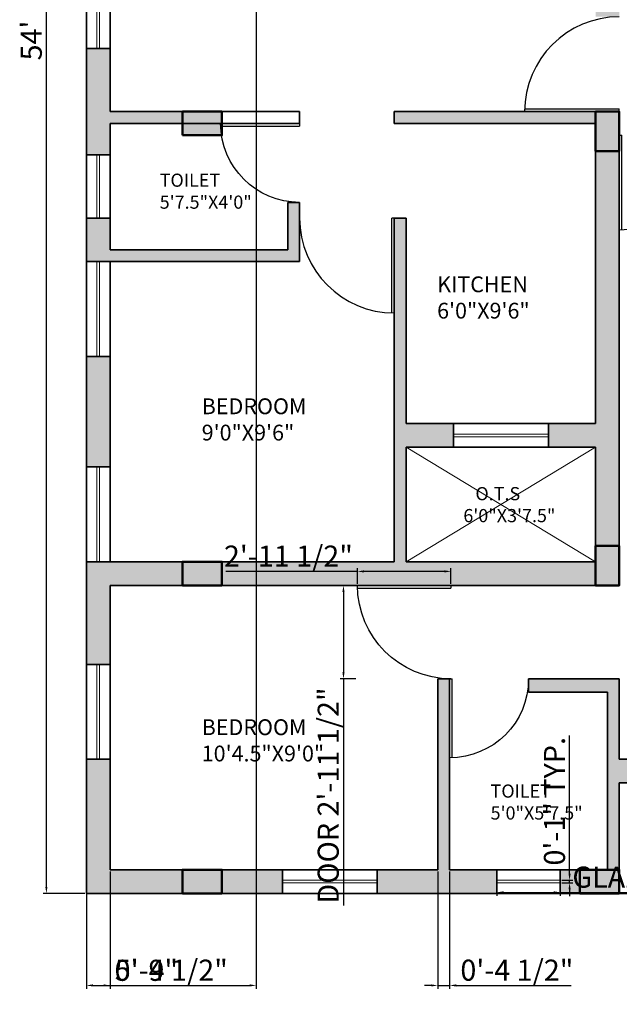
# Model space of a CAD drawing. Units: inches. Extents: x 3010 to 3575, y 2253 to 2995.
# Tile 1 of 4: x 3030 to 3258, y 2253 to 2627. Entities that reach past the tile are written whole.
import ezdxf

# ---------------------------------------------------------------- set-up
doc = ezdxf.new("R2010")
doc.units = ezdxf.units.IN
for name, color, linetype, lineweight in [('A-ANNO-DIMS', 2, 'Continuous', 18), ('A-AREA-IDEN', 7, 'Continuous', 18), ('A-COLS', 7, 'Continuous', 50), ('A-COLS-PATT', 1, 'Continuous', 13), ('A-DOOR', 3, 'Continuous', 25), ('A-FLOR-OPEN', 8, 'Continuous', 18), ('A-GLAZ', 4, 'Continuous', 18), ('A-WALL', 7, 'Continuous', 35)]:
    doc.layers.add(name, color=color, linetype=linetype, lineweight=lineweight)
doc.layers.add('A-WALL-PATT', color=9, linetype='Continuous', lineweight=13, true_color=0xc7c8ca)
doc.styles.get("Standard").update_dxf_attribs({"font": 'arial.ttf'})
doc.dimstyles.new('ISO-25', dxfattribs={"dimtxt": 8, "dimasz": 2.5, "dimexe": 1.25, "dimexo": 0.625, "dimtad": 1, "dimdec": 1, "dimlunit": 3, "dimtxsty": 'Standard', "dimcen": 2.5, "dimadec": 0, "dimazin": 0, "dimtfac": 1, "dimtdec": 1, "dimtmove": 0, "dimatfit": 3, "dimfxl": 1, "dimarcsym": 0})

# ---------------------------------------------------------------- blocks, each defined once
blk = doc.blocks.new('*D2')
at = {"layer": 'A-ANNO-DIMS', "color": 0, "lineweight": -2, "transparency": 16777216}
for p, q in [((3054.82, 2943.38), (3038.98, 2943.38)), ((3040.23, 2297.88), (3040.23, 2940.88)), ((3054.82, 2295.38), (3038.98, 2295.38))]:
    blk.add_line(p, q, dxfattribs=at)
at = {"layer": 'A-ANNO-DIMS', "color": 0, "transparency": 16777216}
for points in [[(3039.81, 2940.88), (3040.64, 2940.88), (3040.23, 2943.38)], [(3039.81, 2297.88), (3040.64, 2297.88), (3040.23, 2295.38)]]:
    blk.add_solid(points, dxfattribs=at)
at = {"layer": 'Defpoints', "color": 0, "transparency": 16777216}
for p in [(3040.23, 2943.38), (3055.45, 2943.38), (3055.45, 2295.38)]:
    blk.add_point(p, dxfattribs=at)
at = {"layer": 'A-ANNO-DIMS', "color": 0, "transparency": 16777216, "insert": (3035.53, 2619.38), "char_height": 8, "attachment_point": 5, "rotation": 90}
blk.add_mtext("54'", dxfattribs=at)
blk = doc.blocks.new("D2 2'6")
for p, q in [((0, 30), (0, 0)), ((1, 30), (1, 0)), ((0, 0), (1, 0))]:
    blk.add_line(p, q)
blk.add_arc((0, 0), 30, 0, 90)
blk = doc.blocks.new("D1 3'")
for p, q in [((0, 36), (0, 0)), ((1, 36), (1, 0)), ((0, 0), (1, 0))]:
    blk.add_line(p, q)
blk.add_arc((0, 0), 36, 0, 90)
blk = doc.blocks.new('1')
for p, q in [((3554.8, 2642.98), (3554.8, 2607.48)), ((3555.8, 2642.97), (3555.8, 2607.48)), ((3554.8, 2607.48), (3555.8, 2607.48))]:
    blk.add_line(p, q)
blk.add_arc((3554.8, 2607.48), 35.5, 0, 90)
blk = doc.blocks.new('GLAZING-24IN')
for p, q in [((24, 1), (0, 1)), ((24, 0), (0, 0))]:
    blk.add_line(p, q)
blk = doc.blocks.new('GLAZING-36IN')
for p, q in [((36, 1), (0, 1)), ((36, 0), (0, 0))]:
    blk.add_line(p, q)
blk = doc.blocks.new('GLAZING-60IN')
for p, q in [((0, 0), (0, 60)), ((1, 0), (1, 60))]:
    blk.add_line(p, q)
blk = doc.blocks.new('*D17')
at = {"layer": 'A-ANNO-DIMS', "color": 0, "lineweight": -2, "transparency": 16777216}
for p, q in [((3211.45, 2298.76), (3211.45, 2294.53)), ((3235.45, 2298.76), (3235.45, 2294.53)), ((3213.95, 2295.78), (3232.95, 2295.78)), ((3235.45, 2295.78), (3323.23, 2295.78))]:
    blk.add_line(p, q, dxfattribs=at)
at = {"layer": 'A-ANNO-DIMS', "color": 0, "transparency": 16777216}
for points in [[(3213.95, 2296.2), (3213.95, 2295.37), (3211.45, 2295.78)], [(3232.95, 2296.2), (3232.95, 2295.37), (3235.45, 2295.78)]]:
    blk.add_solid(points, dxfattribs=at)
at = {"layer": 'Defpoints', "color": 0, "transparency": 16777216}
for p in [(3211.45, 2299.38), (3235.45, 2299.38), (3235.45, 2295.78)]:
    blk.add_point(p, dxfattribs=at)
at = {"layer": 'A-ANNO-DIMS', "color": 0, "transparency": 16777216, "insert": (3280.59, 2300.54), "char_height": 8, "attachment_point": 5}
blk.add_mtext('GLAZ. 2\'-0" TYP.', dxfattribs=at)
blk = doc.blocks.new('*D18')
at = {"layer": 'A-ANNO-DIMS', "color": 0, "lineweight": -2, "transparency": 16777216}
for p, q in [((3239.05, 2302.88), (3239.05, 2355.4)), ((3236.07, 2300.38), (3240.3, 2300.38)), ((3239.05, 2299.38), (3239.05, 2300.38)), ((3236.07, 2299.38), (3240.3, 2299.38)), ((3239.05, 2296.88), (3239.05, 2294.38))]:
    blk.add_line(p, q, dxfattribs=at)
at = {"layer": 'A-ANNO-DIMS', "color": 0, "transparency": 16777216}
for points in [[(3238.63, 2302.88), (3239.46, 2302.88), (3239.05, 2300.38)], [(3238.63, 2296.88), (3239.46, 2296.88), (3239.05, 2299.38)]]:
    blk.add_solid(points, dxfattribs=at)
at = {"layer": 'Defpoints', "color": 0, "transparency": 16777216}
for p in [(3235.45, 2300.38), (3239.05, 2300.38), (3235.45, 2299.38)]:
    blk.add_point(p, dxfattribs=at)
at = {"layer": 'A-ANNO-DIMS', "color": 0, "transparency": 16777216, "insert": (3234.34, 2330.39), "char_height": 8, "attachment_point": 5, "rotation": 90}
blk.add_mtext('0\'-1" TYP.', dxfattribs=at)
blk = doc.blocks.new('*D27')
at = {"layer": 'A-ANNO-DIMS', "color": 0, "lineweight": -2, "transparency": 16777216}
for p, q in [((3157.82, 2412.38), (3151.87, 2412.38)), ((3153.12, 2409.88), (3153.12, 2379.38)), ((3157.82, 2376.88), (3151.87, 2376.88)), ((3153.12, 2376.88), (3153.12, 2290.78))]:
    blk.add_line(p, q, dxfattribs=at)
at = {"layer": 'A-ANNO-DIMS', "color": 0, "transparency": 16777216}
for points in [[(3152.7, 2409.88), (3153.54, 2409.88), (3153.12, 2412.38)], [(3152.7, 2379.38), (3153.54, 2379.38), (3153.12, 2376.88)]]:
    blk.add_solid(points, dxfattribs=at)
at = {"layer": 'Defpoints', "color": 0, "transparency": 16777216}
for p in [(3158.45, 2412.38), (3153.12, 2376.88), (3158.45, 2376.88)]:
    blk.add_point(p, dxfattribs=at)
at = {"layer": 'A-ANNO-DIMS', "color": 0, "transparency": 16777216, "insert": (3148.36, 2332.58), "char_height": 8, "attachment_point": 5, "rotation": 90}
blk.add_mtext('DOOR 2\'-11 1/2"', dxfattribs=at)
blk = doc.blocks.new('*D28')
at = {"layer": 'A-ANNO-DIMS', "color": 0, "lineweight": -2, "transparency": 16777216}
for p, q in [((3158.45, 2417.71), (3108.44, 2417.71)), ((3158.45, 2413.01), (3158.45, 2418.96)), ((3191.45, 2417.71), (3160.95, 2417.71)), ((3193.95, 2413.01), (3193.95, 2418.96))]:
    blk.add_line(p, q, dxfattribs=at)
at = {"layer": 'A-ANNO-DIMS', "color": 0, "transparency": 16777216}
for points in [[(3160.95, 2418.12), (3160.95, 2417.29), (3158.45, 2417.71)], [(3191.45, 2418.12), (3191.45, 2417.29), (3193.95, 2417.71)]]:
    blk.add_solid(points, dxfattribs=at)
at = {"layer": 'Defpoints', "color": 0, "transparency": 16777216}
for p in [(3158.45, 2417.71), (3158.45, 2412.38), (3193.95, 2412.38)]:
    blk.add_point(p, dxfattribs=at)
at = {"layer": 'A-ANNO-DIMS', "color": 0, "transparency": 16777216, "insert": (3132.19, 2422.47), "char_height": 8, "attachment_point": 5}
blk.add_mtext('2\'-11 1/2"', dxfattribs=at)
blk = doc.blocks.new('*D46')
at = {"layer": 'A-ANNO-DIMS', "color": 0, "lineweight": -2, "transparency": 16777216}
for p, q in [((3064.45, 2303.76), (3064.45, 2259.18)), ((3055.45, 2294.76), (3055.45, 2259.18)), ((3057.95, 2260.43), (3061.95, 2260.43)), ((3064.45, 2260.43), (3089.46, 2260.43))]:
    blk.add_line(p, q, dxfattribs=at)
at = {"layer": 'A-ANNO-DIMS', "color": 0, "transparency": 16777216}
for points in [[(3057.95, 2260.85), (3057.95, 2260.02), (3055.45, 2260.43)], [(3061.95, 2260.85), (3061.95, 2260.02), (3064.45, 2260.43)]]:
    blk.add_solid(points, dxfattribs=at)
at = {"layer": 'Defpoints', "color": 0, "transparency": 16777216}
for p in [(3064.45, 2304.38), (3055.45, 2295.38), (3064.45, 2260.43)]:
    blk.add_point(p, dxfattribs=at)
at = {"layer": 'A-ANNO-DIMS', "color": 0, "transparency": 16777216, "insert": (3078.2, 2265.14), "char_height": 8, "attachment_point": 5}
blk.add_mtext('0\'-9"', dxfattribs=at)
blk = doc.blocks.new('*D47')
at = {"layer": 'A-ANNO-DIMS', "color": 0, "lineweight": -2, "transparency": 16777216}
for p, q in [((3188.95, 2303.76), (3188.95, 2259.18)), ((3193.45, 2303.76), (3193.45, 2259.18)), ((3186.45, 2260.43), (3183.95, 2260.43)), ((3188.95, 2260.43), (3193.45, 2260.43)), ((3195.95, 2260.43), (3239.6, 2260.43))]:
    blk.add_line(p, q, dxfattribs=at)
at = {"layer": 'A-ANNO-DIMS', "color": 0, "transparency": 16777216}
for points in [[(3186.45, 2260.85), (3186.45, 2260.02), (3188.95, 2260.43)], [(3195.95, 2260.85), (3195.95, 2260.02), (3193.45, 2260.43)]]:
    blk.add_solid(points, dxfattribs=at)
at = {"layer": 'Defpoints', "color": 0, "transparency": 16777216}
for p in [(3188.95, 2304.38), (3193.45, 2304.38), (3193.45, 2260.43)]:
    blk.add_point(p, dxfattribs=at)
at = {"layer": 'A-ANNO-DIMS', "color": 0, "transparency": 16777216, "insert": (3219.02, 2265.19), "char_height": 8, "attachment_point": 5}
blk.add_mtext('0\'-4 1/2"', dxfattribs=at)
blk = doc.blocks.new('*D53')
at = {"layer": 'A-ANNO-DIMS', "color": 0, "lineweight": -2, "transparency": 16777216}
for p, q in [((3055.45, 2816.76), (3055.45, 2259.18)), ((3119.95, 2816.76), (3119.95, 2259.18)), ((3057.95, 2260.43), (3117.45, 2260.43))]:
    blk.add_line(p, q, dxfattribs=at)
at = {"layer": 'A-ANNO-DIMS', "color": 0, "transparency": 16777216}
for points in [[(3057.95, 2260.85), (3057.95, 2260.02), (3055.45, 2260.43)], [(3117.45, 2260.85), (3117.45, 2260.02), (3119.95, 2260.43)]]:
    blk.add_solid(points, dxfattribs=at)
at = {"layer": 'Defpoints', "color": 0, "transparency": 16777216}
for p in [(3055.45, 2817.38), (3119.95, 2817.38), (3119.95, 2260.43)]:
    blk.add_point(p, dxfattribs=at)
at = {"layer": 'A-ANNO-DIMS', "color": 0, "transparency": 16777216, "insert": (3087.7, 2265.19), "char_height": 8, "attachment_point": 5}
blk.add_mtext('5\'-4 1/2"', dxfattribs=at)

msp = doc.modelspace()

# ---------------------------------------------------------------- hatches: boundary and pattern name
at = {"layer": 'A-COLS-PATT'}
h = msp.add_hatch(color=256, dxfattribs=at)
h.dxf.hatch_style = 1
h.paths.add_polyline_path([(3106.95, 2583.38), (3106.95, 2592.38), (3091.95, 2592.38), (3091.95, 2583.38)])
h = msp.add_hatch(color=256, dxfattribs=at)
h.dxf.hatch_style = 1
h.paths.add_polyline_path([(3248.95, 2577.38), (3257.95, 2577.38), (3257.95, 2592.38), (3248.95, 2592.38)])
h = msp.add_hatch(color=256, dxfattribs=at)
h.dxf.hatch_style = 1
h.paths.add_polyline_path([(3248.95, 2412.38), (3257.95, 2412.38), (3257.95, 2427.38), (3248.95, 2427.38)])
h = msp.add_hatch(color=256, dxfattribs=at)
h.dxf.hatch_style = 1
h.paths.add_polyline_path([(3106.95, 2412.38), (3106.95, 2421.38), (3091.95, 2421.38), (3091.95, 2412.38)])
h = msp.add_hatch(color=256, dxfattribs=at)
h.dxf.hatch_style = 1
h.paths.add_polyline_path([(3106.95, 2295.38), (3106.95, 2304.38), (3091.95, 2304.38), (3091.95, 2295.38)])
h = msp.add_hatch(color=256, dxfattribs=at)
h.dxf.hatch_style = 1
h.paths.add_polyline_path([(3257.95, 2295.38), (3257.95, 2304.38), (3242.95, 2304.38), (3242.95, 2295.38)])
at = {"layer": 'A-WALL-PATT', "transparency": 33554687}
h = msp.add_hatch(color=256, dxfattribs=at)
h.dxf.hatch_style = 1
h.paths.add_polyline_path([(3064.45, 2499.38), (3055.45, 2499.38), (3055.45, 2457.38), (3064.45, 2457.38)])
h.paths.add_polyline_path([(3091.95, 2421.38), (3055.45, 2421.38), (3055.45, 2382.38), (3064.45, 2382.38), (3064.45, 2412.38), (3091.95, 2412.38)])
h.paths.add_polyline_path([(3248.95, 2421.38), (3176.95, 2421.38), (3176.95, 2464.88), (3194.99, 2464.88), (3194.99, 2473.88), (3176.95, 2473.88), (3176.95, 2551.88), (3172.45, 2551.88), (3172.45, 2515.88), (3172.45, 2421.38), (3106.95, 2421.38), (3106.95, 2412.38), (3248.95, 2412.38)])
h.paths.add_polyline_path([(3064.45, 2346.38), (3055.45, 2346.38), (3055.45, 2295.38), (3091.95, 2295.38), (3091.95, 2304.38), (3064.45, 2304.38)])
h.paths.add_polyline_path([(3129.95, 2304.38), (3106.95, 2304.38), (3106.95, 2295.38), (3129.95, 2295.38)])
h.paths.add_polyline_path([(3211.45, 2304.38), (3193.45, 2304.38), (3193.45, 2376.88), (3188.95, 2376.88), (3188.95, 2304.38), (3165.95, 2304.38), (3165.95, 2295.38), (3211.45, 2295.38)])
h.paths.add_polyline_path([(3269.95, 2346.38), (3257.95, 2346.38), (3257.95, 2376.88), (3223.45, 2376.88), (3223.45, 2371.88), (3253.45, 2371.88), (3253.45, 2304.38), (3257.95, 2304.38), (3257.95, 2337.38), (3269.95, 2337.38)])
h.paths.add_polyline_path([(3242.95, 2304.38), (3235.45, 2304.38), (3235.45, 2295.38), (3242.95, 2295.38)])
h.paths.add_polyline_path([(3370.45, 2346.38), (3353.95, 2346.38), (3353.95, 2337.38), (3365.95, 2337.38), (3365.95, 2304.38), (3370.45, 2304.38)])
h.paths.add_polyline_path([(3389.94, 2304.38), (3380.95, 2304.38), (3380.95, 2295.38), (3389.94, 2295.38)], flags=17)
h.paths.add_polyline_path([(3435.95, 2304.38), (3425.94, 2304.38), (3425.94, 2295.38), (3435.95, 2295.38)], flags=17)
h.paths.add_polyline_path([(3487.45, 2401.88), (3478.45, 2401.88), (3478.45, 2389.88), (3394.45, 2389.88), (3394.45, 2442.38), (3380.95, 2442.38), (3380.95, 2437.88), (3389.95, 2437.88), (3389.95, 2389.88), (3365.95, 2389.88), (3365.95, 2385.38), (3412.45, 2385.38), (3412.45, 2373.38), (3416.95, 2373.38), (3416.95, 2385.38), (3478.45, 2385.38), (3478.45, 2304.38), (3450.95, 2304.38), (3450.95, 2295.38), (3487.45, 2295.38)])
h.paths.add_polyline_path([(3487.45, 2478.38), (3478.45, 2478.38), (3478.45, 2442.38), (3450.95, 2442.38), (3450.95, 2437.88), (3478.45, 2437.88), (3478.45, 2425.88), (3487.45, 2425.88)])
h.paths.add_polyline_path([(3435.95, 2442.38), (3424.45, 2442.38), (3424.45, 2437.88), (3435.95, 2437.88)], flags=17)
h.paths.add_polyline_path([(3248.95, 2592.38), (3221.95, 2592.38), (3172.45, 2592.38), (3172.45, 2587.88), (3248.95, 2587.88)])
h.paths.add_polyline_path([(3257.95, 2577.38), (3248.95, 2577.38), (3248.95, 2473.88), (3230.99, 2473.88), (3230.99, 2464.88), (3248.95, 2464.88), (3248.95, 2427.38), (3257.95, 2427.38)])
h.paths.add_polyline_path([(3365.95, 2583.38), (3293.95, 2583.38), (3293.95, 2574.38), (3365.95, 2574.38)])
h.paths.add_polyline_path([(3370.45, 2574.38), (3365.95, 2574.38), (3365.95, 2478.38), (3370.45, 2478.38)])
h.paths.add_polyline_path([(3435.95, 2583.38), (3380.95, 2583.38), (3380.95, 2574.38), (3435.95, 2574.38)])
h.paths.add_polyline_path([(3487.45, 2583.38), (3450.95, 2583.38), (3450.95, 2574.38), (3478.45, 2574.38), (3478.45, 2538.38), (3487.45, 2538.38)])
h.paths.add_polyline_path([(3064.45, 2551.88), (3055.45, 2551.88), (3055.45, 2535.38), (3136.45, 2535.38), (3136.45, 2557.88), (3131.95, 2557.88), (3131.95, 2539.88), (3064.45, 2539.88)])
h.paths.add_polyline_path([(3091.95, 2704.88), (3064.45, 2704.88), (3064.45, 2726.63), (3055.45, 2726.63), (3055.45, 2676.38), (3064.45, 2676.38), (3064.45, 2700.38), (3091.95, 2700.38)])
h.paths.add_polyline_path([(3064.45, 2616.38), (3055.45, 2616.38), (3055.45, 2575.88), (3064.45, 2575.88), (3064.45, 2587.88), (3091.95, 2587.88), (3091.95, 2592.38), (3064.45, 2592.38)])
h.paths.add_polyline_path([(3487.45, 2688.38), (3478.45, 2688.38), (3478.45, 2670.38), (3450.95, 2670.38), (3450.95, 2661.38), (3487.45, 2661.38)])
h.paths.add_polyline_path([(3450.95, 2661.38), (3446.45, 2661.38), (3446.45, 2583.38), (3450.95, 2583.38)])
h.paths.add_polyline_path([(3435.95, 2670.38), (3380.95, 2670.38), (3380.95, 2661.38), (3435.95, 2661.38)])
h.paths.add_polyline_path([(3365.95, 2670.38), (3293.95, 2670.38), (3293.95, 2661.38), (3365.95, 2661.38)])
h.paths.add_polyline_path([(3370.45, 2715.38), (3365.95, 2715.38), (3365.95, 2670.38), (3370.45, 2670.38)])
h.paths.add_polyline_path([(3257.95, 2700.38), (3248.95, 2700.38), (3248.95, 2628.38), (3257.95, 2628.38)])
h.paths.add_polyline_path([(3128.95, 2742.38), (3124.45, 2742.38), (3124.45, 2704.88), (3106.95, 2704.88), (3106.95, 2700.38), (3128.95, 2700.38)])
h.paths.add_polyline_path([(3248.95, 2704.88), (3164.95, 2704.88), (3164.95, 2700.38), (3248.95, 2700.38)])
h.paths.add_polyline_path([(3257.95, 2817.38), (3248.95, 2817.38), (3248.95, 2715.38), (3257.95, 2715.38)])
h.paths.add_polyline_path([(3128.95, 2781.38), (3055.45, 2781.38), (3055.45, 2750.63), (3064.45, 2750.63), (3064.45, 2772.38), (3128.95, 2772.38)])
h.paths.add_polyline_path([(3242.95, 2826.38), (3106.95, 2826.38), (3106.95, 2817.38), (3242.95, 2817.38)])
h.paths.add_polyline_path([(3091.95, 2826.38), (3064.45, 2826.38), (3064.45, 2856.38), (3055.45, 2856.38), (3055.45, 2817.38), (3091.95, 2817.38)])
h.paths.add_polyline_path([(3064.45, 2934.38), (3091.95, 2934.38), (3091.95, 2943.38), (3055.45, 2943.38), (3055.45, 2904.38), (3064.45, 2904.38)])
h.paths.add_polyline_path([(3140.95, 2943.38), (3106.95, 2943.38), (3106.95, 2934.38), (3140.95, 2934.38)])
h.paths.add_polyline_path([(3211.45, 2943.38), (3188.95, 2943.38), (3188.95, 2862.38), (3223.45, 2862.38), (3223.45, 2866.88), (3193.45, 2866.88), (3193.45, 2934.38), (3211.45, 2934.38)])
h.paths.add_polyline_path([(3257.95, 2934.38), (3253.45, 2934.38), (3253.45, 2862.38), (3257.95, 2862.38), (3257.95, 2892.38), (3269.95, 2892.38), (3269.95, 2901.38), (3257.95, 2901.38)])
h.paths.add_polyline_path([(3242.95, 2943.38), (3235.45, 2943.38), (3235.45, 2934.38), (3242.95, 2934.38)])
h.paths.add_polyline_path([(3370.45, 2934.38), (3365.95, 2934.38), (3365.95, 2901.38), (3353.95, 2901.38), (3353.95, 2892.38), (3365.95, 2892.38), (3365.95, 2844.38), (3370.45, 2844.38)])
h.paths.add_polyline_path([(3389.94, 2943.38), (3380.95, 2943.38), (3380.95, 2934.38), (3389.94, 2934.38)])
h.paths.add_polyline_path([(3435.95, 2943.38), (3425.94, 2943.38), (3425.94, 2934.38), (3435.95, 2934.38)])
h.paths.add_polyline_path([(3487.45, 2943.38), (3450.95, 2943.38), (3450.95, 2934.38), (3478.45, 2934.38), (3478.45, 2895.38), (3487.45, 2895.38)])
h.paths.add_polyline_path([(3487.45, 2847.38), (3478.45, 2847.38), (3478.45, 2808.38), (3450.95, 2808.38), (3450.95, 2803.88), (3478.45, 2803.88), (3478.45, 2791.88), (3487.45, 2791.88)])
h.paths.add_polyline_path([(3435.95, 2808.38), (3424.45, 2808.38), (3424.45, 2803.88), (3435.95, 2803.88)])
h.paths.add_polyline_path([(3487.45, 2767.88), (3478.45, 2767.88), (3478.45, 2755.88), (3394.45, 2755.88), (3394.45, 2808.38), (3380.95, 2808.38), (3380.95, 2803.88), (3389.95, 2803.88), (3389.95, 2755.88), (3365.95, 2755.88), (3365.95, 2751.38), (3412.45, 2751.38), (3412.45, 2739.38), (3416.95, 2739.38), (3416.95, 2751.38), (3478.45, 2751.38), (3478.45, 2724.38), (3487.45, 2724.38)])
h.paths.add_polyline_path([(3398.97, 2495.84), (3456.57, 2495.84), (3456.57, 2518.66), (3398.97, 2518.66)], flags=9)

# ---------------------------------------------------------------- linework, layer by layer
at = {"layer": 'A-COLS'}
for points in [[(3091.95, 2583.38), (3091.95, 2592.38), (3106.95, 2592.38), (3106.95, 2583.38)], [(3248.95, 2592.38), (3257.95, 2592.38), (3257.95, 2577.38), (3248.95, 2577.38)], [(3248.95, 2427.38), (3257.95, 2427.38), (3257.95, 2412.38), (3248.95, 2412.38)], [(3091.95, 2412.38), (3091.95, 2421.38), (3106.95, 2421.38), (3106.95, 2412.38)], [(3091.95, 2295.38), (3091.95, 2304.38), (3106.95, 2304.38), (3106.95, 2295.38)], [(3242.95, 2295.38), (3242.95, 2304.38), (3257.95, 2304.38), (3257.95, 2295.38)]]:
    msp.add_lwpolyline(points, close=True, dxfattribs=at)
at = {"layer": 'A-FLOR-OPEN'}
for p, q in [((3176.95, 2464.88), (3248.95, 2421.38)), ((3176.95, 2421.38), (3248.95, 2464.88))]:
    msp.add_line(p, q, dxfattribs=at)
at = {"layer": 'A-WALL'}
for p, q in [((3055.45, 2535.38), (3055.45, 2781.38)), ((3064.45, 2592.38), (3064.45, 2700.38)), ((3064.45, 2616.38), (3055.45, 2616.38)), ((3064.45, 2592.38), (3136.45, 2592.38)), ((3136.45, 2587.88), (3136.45, 2592.38)), ((3172.45, 2592.38), (3257.95, 2592.38)), ((3172.45, 2587.88), (3172.45, 2592.38)), ((3257.95, 2412.38), (3257.95, 2592.38)), ((3064.45, 2587.88), (3136.45, 2587.88)), ((3064.45, 2539.88), (3064.45, 2587.88)), ((3172.45, 2587.88), (3248.95, 2587.88)), ((3248.95, 2473.88), (3248.95, 2587.88)), ((3064.45, 2575.88), (3055.45, 2575.88)), ((3131.95, 2539.88), (3131.95, 2557.88)), ((3131.95, 2557.88), (3136.45, 2557.88)), ((3136.45, 2535.38), (3136.45, 2557.88)), ((3064.45, 2551.88), (3055.45, 2551.88)), ((3172.45, 2421.38), (3172.45, 2551.88)), ((3172.45, 2551.88), (3176.95, 2551.88)), ((3176.95, 2473.88), (3176.95, 2551.88)), ((3064.45, 2539.88), (3131.95, 2539.88)), ((3055.45, 2295.38), (3055.45, 2535.38)), ((3055.45, 2535.38), (3136.45, 2535.38)), ((3064.45, 2421.38), (3064.45, 2535.38)), ((3055.45, 2499.38), (3064.45, 2499.38)), ((3176.95, 2473.88), (3248.95, 2473.88)), ((3194.99, 2473.88), (3194.99, 2464.88)), ((3230.99, 2473.88), (3230.99, 2464.88)), ((3176.95, 2464.88), (3248.95, 2464.88)), ((3176.95, 2421.38), (3176.95, 2464.88)), ((3248.95, 2421.38), (3248.95, 2464.88)), ((3055.45, 2457.38), (3064.45, 2457.38)), ((3055.45, 2421.38), (3172.45, 2421.38)), ((3176.95, 2421.38), (3248.95, 2421.38)), ((3064.45, 2304.38), (3064.45, 2412.38)), ((3064.45, 2412.38), (3257.95, 2412.38)), ((3064.45, 2382.38), (3055.45, 2382.38)), ((3188.95, 2304.38), (3188.95, 2376.88)), ((3193.45, 2376.88), (3188.95, 2376.88)), ((3193.45, 2304.38), (3193.45, 2376.88)), ((3257.95, 2376.88), (3223.45, 2376.88)), ((3223.45, 2371.88), (3223.45, 2376.88)), ((3257.95, 2346.38), (3257.95, 2376.88)), ((3253.45, 2371.88), (3223.45, 2371.88)), ((3253.45, 2304.38), (3253.45, 2371.88)), ((3064.45, 2346.38), (3055.45, 2346.38)), ((3269.95, 2346.38), (3257.95, 2346.38)), ((3257.95, 2295.38), (3257.95, 2337.38)), ((3269.95, 2337.38), (3257.95, 2337.38)), ((3188.95, 2304.38), (3064.45, 2304.38)), ((3129.95, 2304.38), (3129.95, 2295.38)), ((3165.95, 2304.38), (3165.95, 2295.38)), ((3253.45, 2304.38), (3193.45, 2304.38)), ((3211.45, 2304.38), (3211.45, 2295.38)), ((3235.45, 2304.38), (3235.45, 2295.38)), ((3487.45, 2295.38), (3055.45, 2295.38))]:
    msp.add_line(p, q, dxfattribs=at)

# ---------------------------------------------------------------- block references
at = {"layer": 'A-DOOR'}
for p, rotation in [((3257.95, 2592.38), 90), ((3172.45, 2551.88), 180)]:
    msp.add_blockref("D1 3'", p, dxfattribs=dict(at, rotation=rotation))
at = {"layer": 'A-DOOR', "xscale": -1}
for name, p, rotation in [("D2 2'6", (3136.45, 2587.88), 90), ("D1 3'", (3257.95, 2583.38), 180), ('1', (5801.43, 5967.19), 90), ("D2 2'6", (3193.45, 2376.88), 180)]:
    msp.add_blockref(name, p, dxfattribs=dict(at, rotation=rotation))
at = {"layer": 'A-GLAZ'}
for name, p in [('GLAZING-60IN', (3059.45, 2616.38)), ('GLAZING-36IN', (3194.99, 2468.88)), ('GLAZING-36IN', (3129.95, 2299.38)), ('GLAZING-24IN', (3211.45, 2299.38))]:
    msp.add_blockref(name, p, dxfattribs=at)
for name, p, rotation in [('GLAZING-24IN', (3059.45, 2575.88), 270), ('GLAZING-36IN', (3059.45, 2535.38), 269.9999999999986), ('GLAZING-36IN', (3059.45, 2457.38), 269.9999999999985), ('GLAZING-36IN', (3059.45, 2382.38), 269.9999999999986)]:
    msp.add_blockref(name, p, dxfattribs=dict(at, rotation=rotation))

# ---------------------------------------------------------------- texts
at = {"layer": 'A-AREA-IDEN', "attachment_point": 1}
for s, insert, char_height in [('{\\fTimes New Roman|b0|i0|c0|p18;\\P  TOILET\\P  5\'7.5"X4\'0"}', (3080.23, 2577.14), 5), ('{\\fTimes New Roman|b0|i0|c0|p18;\\PKITCHEN\\P6\'0"X9\'6"}', (3188.7, 2539.75), 6), ('{\\fTimes New Roman|b0|i0|c0|p18;\\PBEDROOM \\P9\'0"X9\'6"}', (3099.24, 2493.43), 6), ('{\\fTimes New Roman|b0|i0|c0|p18;\\P     O.T.S\\P  6\'0"X3\'7.5"}', (3195.62, 2458.07), 5), ('{\\fTimes New Roman|b0|i0|c0|p18;\\PBEDROOM \\P10\'4.5"X9\'0"}', (3099.24, 2371.53), 6), ('{\\fTimes New Roman|b0|i0|c0|p18;\\P  TOILET\\P  5\'0"X5\'7.5"}', (3205.97, 2345.1), 5)]:
    msp.add_mtext_dynamic_manual_height_columns(s, width=72.5587, gutter_width=12.5, heights=[0], dxfattribs=dict(at, insert=insert, char_height=char_height))

# ---------------------------------------------------------------- dimensions: what is measured, and where the dimension line sits
at = {"layer": 'A-ANNO-DIMS'}
for base, p1, p2, angle, override, picture, middle in [((3040.23, 2943.38), (3055.45, 2295.38), (3055.45, 2943.38), 270, {"dimclrd": 0, "dimclre": 0, "dimclrt": 0}, '*D2', (3035.53, 2619.38)), ((3158.45, 2417.71), (3193.95, 2412.38), (3158.45, 2412.38), 180, {"dimdec": 1, "dimlfac": 1, "dimrnd": 0, "dimzin": 1, "dimdsep": 46, "dimlunit": 4, "dimfrac": 2}, '*D28', (3132.19, 2422.47))]:
    dim = msp.add_linear_dim(base=base, p1=p1, p2=p2, angle=angle, dimstyle='ISO-25', override=override, dxfattribs=at)
    dim.commit()
    dim.dimension.update_dxf_attribs({"geometry": picture, "text_midpoint": middle})
for base, p1, p2, picture, middle in [((3119.95, 2260.43), (3055.45, 2817.38), (3119.95, 2817.38), '*D53', (3087.7, 2265.19)), ((3064.45, 2260.43), (3055.45, 2295.38), (3064.45, 2304.38), '*D46', (3078.2, 2265.14)), ((3193.45, 2260.43), (3188.95, 2304.38), (3193.45, 2304.38), '*D47', (3219.02, 2265.19))]:
    dim = msp.add_linear_dim(base=base, p1=p1, p2=p2, dimstyle='ISO-25', override={"dimdec": 1, "dimlfac": 1, "dimrnd": 0, "dimzin": 1, "dimdsep": 46, "dimlunit": 4, "dimfrac": 2}, dxfattribs=at)
    dim.commit()
    dim.dimension.update_dxf_attribs({"geometry": picture, "text_midpoint": middle})
for base, p1, p2, angle, text, picture, middle in [((3153.12, 2376.88), (3158.45, 2412.38), (3158.45, 2376.88), 270, 'DOOR <>', '*D27', (3148.36, 2332.58)), ((3239.05, 2300.38), (3235.45, 2299.38), (3235.45, 2300.38), 90, '<> TYP.', '*D18', (3234.34, 2330.39))]:
    dim = msp.add_linear_dim(base=base, p1=p1, p2=p2, angle=angle, text=text, dimstyle='ISO-25', override={"dimdec": 1, "dimlfac": 1, "dimrnd": 0, "dimzin": 1, "dimdsep": 46, "dimlunit": 4, "dimfrac": 2}, dxfattribs=at)
    dim.commit()
    dim.dimension.update_dxf_attribs({"geometry": picture, "text_midpoint": middle})
dim = msp.add_linear_dim(base=(3235.45, 2295.78), p1=(3211.45, 2299.38), p2=(3235.45, 2299.38), text='GLAZ. <> TYP.', dimstyle='ISO-25', override={"dimdec": 1, "dimlfac": 1, "dimrnd": 0, "dimzin": 1, "dimdsep": 46, "dimlunit": 4, "dimfrac": 2}, dxfattribs=at)
dim.commit()
dim.dimension.update_dxf_attribs({"geometry": '*D17', "text_midpoint": (3280.59, 2300.54)})

doc.saveas('drawing.dxf')
